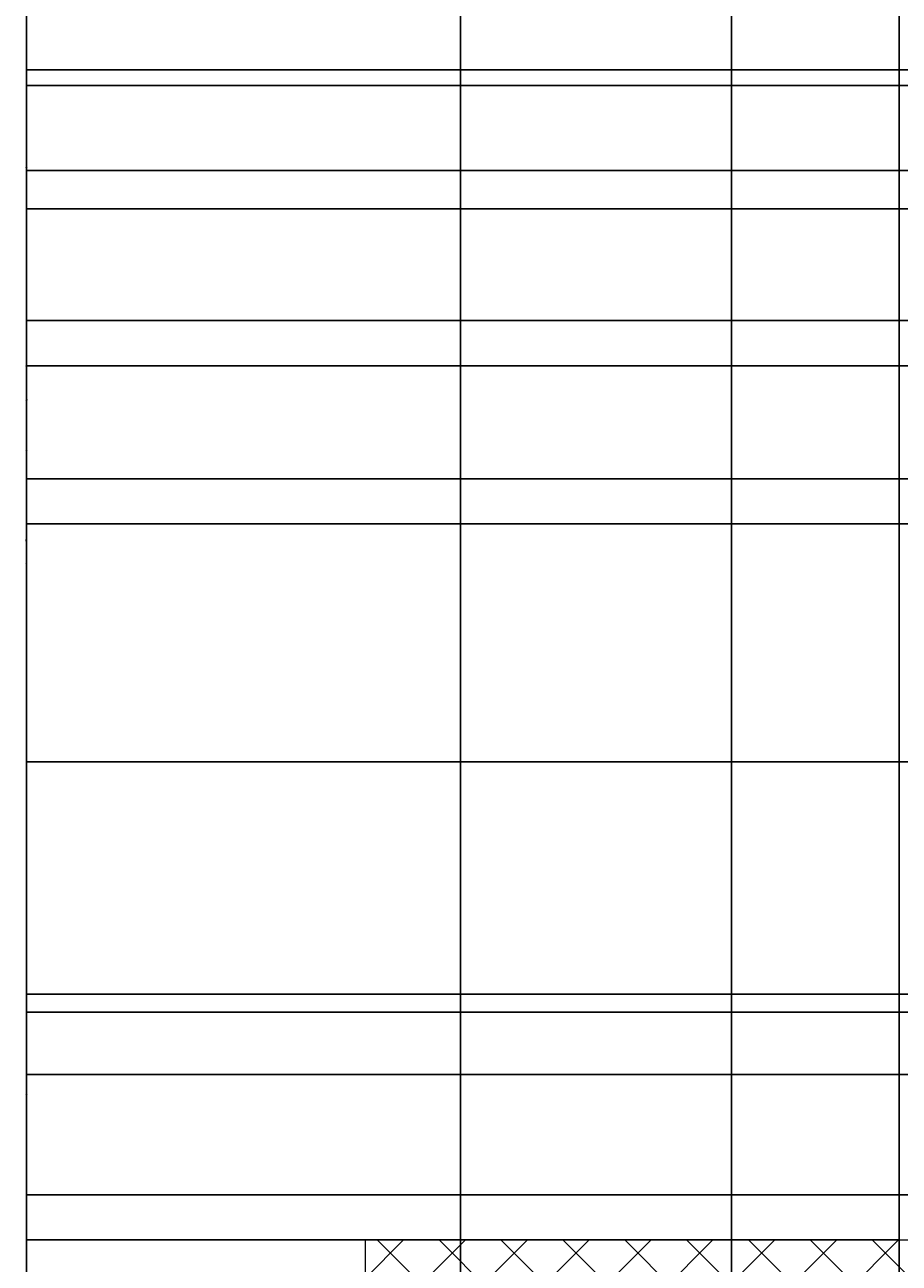
# Model space of a CAD drawing. Units: inches. Extents: x 818 to 1898, y 976 to 2364.
# Tile 2 of 96: x 818 to 993, y 1198 to 1446. Entities that reach past the tile are written whole.
import ezdxf

# ---------------------------------------------------------------- set-up
doc = ezdxf.new("R2010")
doc.units = ezdxf.units.IN
doc.header["$LTSCALE"] = 5
doc.header["$MEASUREMENT"] = 0
for name, color, linetype, lineweight in [('A-ANNO-DIMS', 2, 'Continuous', 18), ('C-PAVE-PATT', 8, 'Continuous', 9), ('L-PAVE', 8, 'Continuous', 18)]:
    doc.layers.add(name, color=color, linetype=linetype, lineweight=lineweight)
doc.styles.get("Standard").update_dxf_attribs({"font": 'arial.ttf'})
doc.dimstyles.get("Standard").update_dxf_attribs({"dimtxt": 0.18, "dimasz": 0.18, "dimexe": 0.18, "dimexo": 0.0625, "dimgap": 0.09, "dimtad": 0, "dimtih": 1, "dimtoh": 1, "dimdec": 4, "dimzin": 0, "dimdsep": 46, "dimtxsty": 'Standard', "dimcen": 0.09, "dimadec": 0, "dimazin": 0, "dimtfac": 1, "dimtdec": 4, "dimtofl": 0, "dimtmove": 0, "dimatfit": 3, "dimfxl": 1, "dimtolj": 1, "dimtzin": 0, "dimarcsym": 0})

# ---------------------------------------------------------------- blocks, each defined once
blk = doc.blocks.new('*D59')
at = {"layer": 'A-ANNO-DIMS', "color": 0, "lineweight": -2, "ltscale": 5, "transparency": 16777216}
for p, q in [((1251.64, 2300.39), (818.03, 2300.39)), ((818.21, 2300.21), (818.21, 1669.95)), ((818.21, 1039.32), (818.21, 1669.59)), ((896.05, 1039.14), (818.03, 1039.14))]:
    blk.add_line(p, q, dxfattribs=at)
at = {"layer": 'A-ANNO-DIMS', "color": 0, "ltscale": 5, "transparency": 16777216}
for points in [[(818.18, 2300.21), (818.24, 2300.21), (818.21, 2300.39)], [(818.18, 1039.32), (818.24, 1039.32), (818.21, 1039.14)]]:
    blk.add_solid(points, dxfattribs=at)
at = {"layer": 'Defpoints', "color": 0, "ltscale": 5, "transparency": 16777216}
for p in [(818.21, 2300.39), (1251.71, 2300.39), (896.11, 1039.14)]:
    blk.add_point(p, dxfattribs=at)
at = {"layer": 'A-ANNO-DIMS', "color": 0, "ltscale": 5, "transparency": 16777216, "insert": (818.21, 1669.77), "char_height": 0.18, "attachment_point": 5}
blk.add_mtext('\\A1;1261.2', dxfattribs=at)
blk = doc.blocks.new('*D60')
at = {"layer": 'A-ANNO-DIMS', "color": 0, "lineweight": -2, "ltscale": 5, "transparency": 16777216}
for p, q in [((992.66, 2294.22), (818.03, 2294.22)), ((818.21, 2294.04), (818.21, 1748.77)), ((818.21, 1203.14), (818.21, 1748.41)), ((992.66, 1202.96), (818.03, 1202.96))]:
    blk.add_line(p, q, dxfattribs=at)
at = {"layer": 'A-ANNO-DIMS', "color": 0, "ltscale": 5, "transparency": 16777216}
for points in [[(818.18, 2294.04), (818.24, 2294.04), (818.21, 2294.22)], [(818.18, 1203.14), (818.24, 1203.14), (818.21, 1202.96)]]:
    blk.add_solid(points, dxfattribs=at)
at = {"layer": 'Defpoints', "color": 0, "ltscale": 5, "transparency": 16777216}
for p in [(818.21, 2294.22), (992.73, 2294.22), (992.73, 1202.96)]:
    blk.add_point(p, dxfattribs=at)
at = {"layer": 'A-ANNO-DIMS', "color": 0, "ltscale": 5, "transparency": 16777216, "insert": (818.21, 1748.59), "char_height": 0.18, "attachment_point": 5}
blk.add_mtext('\\A1;1091.3', dxfattribs=at)
blk = doc.blocks.new('*D63')
at = {"layer": 'A-ANNO-DIMS', "color": 0, "lineweight": -2, "ltscale": 5, "transparency": 16777216}
for p, q in [((1116.13, 1485.2), (818.03, 1485.2)), ((818.21, 1485.02), (818.21, 1360.77)), ((818.21, 1236.14), (818.21, 1360.4)), ((1116.13, 1235.96), (818.03, 1235.96))]:
    blk.add_line(p, q, dxfattribs=at)
at = {"layer": 'A-ANNO-DIMS', "color": 0, "ltscale": 5, "transparency": 16777216}
for points in [[(818.18, 1485.02), (818.24, 1485.02), (818.21, 1485.2)], [(818.18, 1236.14), (818.24, 1236.14), (818.21, 1235.96)]]:
    blk.add_solid(points, dxfattribs=at)
at = {"layer": 'Defpoints', "color": 0, "ltscale": 5, "transparency": 16777216}
for p in [(818.21, 1485.2), (1116.19, 1485.2), (1116.19, 1235.96)]:
    blk.add_point(p, dxfattribs=at)
at = {"layer": 'A-ANNO-DIMS', "color": 0, "ltscale": 5, "transparency": 16777216, "insert": (818.21, 1360.58), "char_height": 0.18, "attachment_point": 5}
blk.add_mtext('\\A1;249.24', dxfattribs=at)
blk = doc.blocks.new('*D77')
at = {"layer": 'A-ANNO-DIMS', "color": 0, "lineweight": -2, "ltscale": 5, "transparency": 16777216}
for p, q in [((992.73, 1202.9), (992.73, 975.66)), ((896.11, 1104.9), (896.11, 975.66)), ((896.29, 975.84), (944.04, 975.84)), ((992.55, 975.84), (944.8, 975.84))]:
    blk.add_line(p, q, dxfattribs=at)
at = {"layer": 'A-ANNO-DIMS', "color": 0, "ltscale": 5, "transparency": 16777216}
for points in [[(896.29, 975.87), (896.29, 975.81), (896.11, 975.84)], [(992.55, 975.87), (992.55, 975.81), (992.73, 975.84)]]:
    blk.add_solid(points, dxfattribs=at)
at = {"layer": 'Defpoints', "color": 0, "ltscale": 5, "transparency": 16777216}
for p in [(992.73, 1202.96), (896.11, 1104.97), (992.73, 975.84)]:
    blk.add_point(p, dxfattribs=at)
at = {"layer": 'A-ANNO-DIMS', "color": 0, "ltscale": 5, "transparency": 16777216, "insert": (944.42, 975.84), "char_height": 0.18, "attachment_point": 5}
blk.add_mtext('\\A1;96.61', dxfattribs=at)
blk = doc.blocks.new('*D79')
at = {"layer": 'A-ANNO-DIMS', "color": 0, "lineweight": -2, "ltscale": 5, "transparency": 16777216}
for p, q in [((992.73, 1203.03), (992.73, 2363.87)), ((992.91, 2363.69), (1032.01, 2363.69)), ((1071.55, 2363.69), (1032.44, 2363.69)), ((1071.73, 1203.03), (1071.73, 2363.87))]:
    blk.add_line(p, q, dxfattribs=at)
at = {"layer": 'A-ANNO-DIMS', "color": 0, "ltscale": 5, "transparency": 16777216}
for points in [[(992.91, 2363.72), (992.91, 2363.66), (992.73, 2363.69)], [(1071.55, 2363.72), (1071.55, 2363.66), (1071.73, 2363.69)]]:
    blk.add_solid(points, dxfattribs=at)
at = {"layer": 'Defpoints', "color": 0, "ltscale": 5, "transparency": 16777216}
for p in [(1071.73, 2363.69), (992.73, 1202.96), (1071.73, 1202.96)]:
    blk.add_point(p, dxfattribs=at)
at = {"layer": 'A-ANNO-DIMS', "color": 0, "ltscale": 5, "transparency": 16777216, "insert": (1032.23, 2363.69), "char_height": 0.18, "attachment_point": 5}
blk.add_mtext('\\A1;79', dxfattribs=at)
blk = doc.blocks.new('*D81')
at = {"layer": 'A-ANNO-DIMS', "color": 0, "lineweight": -2, "ltscale": 5, "transparency": 16777216}
for p, q in [((1116.13, 1235.96), (818.03, 1235.96)), ((818.21, 1235.78), (818.21, 1224.14)), ((818.21, 1212.14), (818.21, 1223.78)), ((1083.66, 1211.96), (818.03, 1211.96))]:
    blk.add_line(p, q, dxfattribs=at)
at = {"layer": 'A-ANNO-DIMS', "color": 0, "ltscale": 5, "transparency": 16777216}
for points in [[(818.18, 1235.78), (818.24, 1235.78), (818.21, 1235.96)], [(818.18, 1212.14), (818.24, 1212.14), (818.21, 1211.96)]]:
    blk.add_solid(points, dxfattribs=at)
at = {"layer": 'Defpoints', "color": 0, "ltscale": 5, "transparency": 16777216}
for p in [(1116.19, 1235.96), (818.21, 1211.96), (1083.73, 1211.96)]:
    blk.add_point(p, dxfattribs=at)
at = {"layer": 'A-ANNO-DIMS', "color": 0, "ltscale": 5, "transparency": 16777216, "insert": (818.21, 1223.96), "char_height": 0.18, "attachment_point": 5}
blk.add_mtext('\\A1;24', dxfattribs=at)
blk = doc.blocks.new('*D90')
at = {"layer": 'A-ANNO-DIMS', "color": 0, "lineweight": -2, "ltscale": 5, "transparency": 16777216}
for p, q in [((904.95, 1071.12), (904.95, 2363.87)), ((905.13, 2363.69), (931.67, 2363.69)), ((958.99, 2363.69), (932.45, 2363.69)), ((959.17, 1071.12), (959.17, 2363.87))]:
    blk.add_line(p, q, dxfattribs=at)
at = {"layer": 'A-ANNO-DIMS', "color": 0, "ltscale": 5, "transparency": 16777216}
for points in [[(905.13, 2363.72), (905.13, 2363.66), (904.95, 2363.69)], [(958.99, 2363.72), (958.99, 2363.66), (959.17, 2363.69)]]:
    blk.add_solid(points, dxfattribs=at)
at = {"layer": 'Defpoints', "color": 0, "ltscale": 5, "transparency": 16777216}
for p in [(959.17, 2363.69), (904.95, 1071.06), (959.17, 1071.06)]:
    blk.add_point(p, dxfattribs=at)
at = {"layer": 'A-ANNO-DIMS', "color": 0, "ltscale": 5, "transparency": 16777216, "insert": (932.06, 2363.69), "char_height": 0.18, "attachment_point": 5}
blk.add_mtext('\\A1;54.22', dxfattribs=at)
blk = doc.blocks.new('*D91')
at = {"layer": 'A-ANNO-DIMS', "color": 0, "lineweight": -2, "ltscale": 5, "transparency": 16777216}
for p, q in [((959.17, 1071.12), (959.17, 2363.87)), ((959.35, 2363.69), (985.8, 2363.69)), ((1013.04, 2363.69), (986.59, 2363.69)), ((1013.22, 1071.12), (1013.22, 2363.87))]:
    blk.add_line(p, q, dxfattribs=at)
at = {"layer": 'A-ANNO-DIMS', "color": 0, "ltscale": 5, "transparency": 16777216}
for points in [[(959.35, 2363.72), (959.35, 2363.66), (959.17, 2363.69)], [(1013.04, 2363.72), (1013.04, 2363.66), (1013.22, 2363.69)]]:
    blk.add_solid(points, dxfattribs=at)
at = {"layer": 'Defpoints', "color": 0, "ltscale": 5, "transparency": 16777216}
for p in [(1013.22, 2363.69), (959.17, 1071.06), (1013.22, 1071.06)]:
    blk.add_point(p, dxfattribs=at)
at = {"layer": 'A-ANNO-DIMS', "color": 0, "ltscale": 5, "transparency": 16777216, "insert": (986.2, 2363.69), "char_height": 0.18, "attachment_point": 5}
blk.add_mtext('\\A1;54.04', dxfattribs=at)
blk = doc.blocks.new('*D108')
at = {"layer": 'A-ANNO-DIMS', "color": 0, "lineweight": -2, "ltscale": 5, "transparency": 16777216}
for p, q in [((1131.74, 1436.86), (818.03, 1436.86)), ((818.21, 1436.68), (818.21, 1342.84)), ((818.21, 1248.64), (818.21, 1342.48)), ((1164.49, 1248.46), (818.03, 1248.46))]:
    blk.add_line(p, q, dxfattribs=at)
at = {"layer": 'A-ANNO-DIMS', "color": 0, "ltscale": 5, "transparency": 16777216}
for points in [[(818.18, 1436.68), (818.24, 1436.68), (818.21, 1436.86)], [(818.18, 1248.64), (818.24, 1248.64), (818.21, 1248.46)]]:
    blk.add_solid(points, dxfattribs=at)
at = {"layer": 'Defpoints', "color": 0, "ltscale": 5, "transparency": 16777216}
for p in [(818.21, 1436.86), (1131.8, 1436.86), (1164.56, 1248.46)]:
    blk.add_point(p, dxfattribs=at)
at = {"layer": 'A-ANNO-DIMS', "color": 0, "ltscale": 5, "transparency": 16777216, "insert": (818.21, 1342.66), "char_height": 0.18, "attachment_point": 5}
blk.add_mtext('\\A1;188.4', dxfattribs=at)
blk = doc.blocks.new('*D115')
at = {"layer": 'A-ANNO-DIMS', "color": 0, "lineweight": -2, "ltscale": 5, "transparency": 16777216}
for p, q in [((1766.29, 1377.66), (818.03, 1377.66)), ((818.21, 1377.48), (818.21, 1338.26)), ((818.21, 1298.68), (818.21, 1337.9)), ((1766.29, 1298.5), (818.03, 1298.5))]:
    blk.add_line(p, q, dxfattribs=at)
at = {"layer": 'A-ANNO-DIMS', "color": 0, "ltscale": 5, "transparency": 16777216}
for points in [[(818.18, 1377.48), (818.24, 1377.48), (818.21, 1377.66)], [(818.18, 1298.68), (818.24, 1298.68), (818.21, 1298.5)]]:
    blk.add_solid(points, dxfattribs=at)
at = {"layer": 'Defpoints', "color": 0, "ltscale": 5, "transparency": 16777216}
for p in [(818.21, 1377.66), (1766.35, 1377.66), (1766.35, 1298.5)]:
    blk.add_point(p, dxfattribs=at)
at = {"layer": 'A-ANNO-DIMS', "color": 0, "ltscale": 5, "transparency": 16777216, "insert": (818.21, 1338.08), "char_height": 0.18, "attachment_point": 5}
blk.add_mtext('\\A1;79.15', dxfattribs=at)
blk = doc.blocks.new('*D116')
at = {"layer": 'A-ANNO-DIMS', "color": 0, "lineweight": -2, "ltscale": 5, "transparency": 16777216}
for p, q in [((1766.29, 1456.81), (818.03, 1456.81)), ((818.21, 1456.63), (818.21, 1417.41)), ((818.21, 1377.84), (818.21, 1417.05)), ((1766.29, 1377.66), (818.03, 1377.66))]:
    blk.add_line(p, q, dxfattribs=at)
at = {"layer": 'A-ANNO-DIMS', "color": 0, "ltscale": 5, "transparency": 16777216}
for points in [[(818.18, 1456.63), (818.24, 1456.63), (818.21, 1456.81)], [(818.18, 1377.84), (818.24, 1377.84), (818.21, 1377.66)]]:
    blk.add_solid(points, dxfattribs=at)
at = {"layer": 'Defpoints', "color": 0, "ltscale": 5, "transparency": 16777216}
for p in [(818.21, 1456.81), (1766.35, 1456.81), (1766.35, 1377.66)]:
    blk.add_point(p, dxfattribs=at)
at = {"layer": 'A-ANNO-DIMS', "color": 0, "ltscale": 5, "transparency": 16777216, "insert": (818.21, 1417.23), "char_height": 0.18, "attachment_point": 5}
blk.add_mtext('\\A1;79.15', dxfattribs=at)
blk = doc.blocks.new('*D127')
at = {"layer": 'A-ANNO-DIMS', "color": 0, "lineweight": -2, "ltscale": 5, "transparency": 16777216}
for p, q in [((1035.31, 1252.02), (818.03, 1252.02)), ((818.21, 1251.84), (818.21, 1232.18)), ((818.21, 1212.14), (818.21, 1231.81)), ((1001.66, 1211.96), (818.03, 1211.96))]:
    blk.add_line(p, q, dxfattribs=at)
at = {"layer": 'A-ANNO-DIMS', "color": 0, "ltscale": 5, "transparency": 16777216}
for points in [[(818.18, 1251.84), (818.24, 1251.84), (818.21, 1252.02)], [(818.18, 1212.14), (818.24, 1212.14), (818.21, 1211.96)]]:
    blk.add_solid(points, dxfattribs=at)
at = {"layer": 'Defpoints', "color": 0, "ltscale": 5, "transparency": 16777216}
for p in [(818.21, 1252.02), (1035.38, 1252.02), (1001.73, 1211.96)]:
    blk.add_point(p, dxfattribs=at)
at = {"layer": 'A-ANNO-DIMS', "color": 0, "ltscale": 5, "transparency": 16777216, "insert": (818.21, 1231.99), "char_height": 0.18, "attachment_point": 5}
blk.add_mtext('\\A1;40.06', dxfattribs=at)
blk = doc.blocks.new('*D128')
at = {"layer": 'A-ANNO-DIMS', "color": 0, "lineweight": -2, "ltscale": 5, "transparency": 16777216}
for p, q in [((1044.78, 1433.67), (818.03, 1433.67)), ((818.21, 1433.49), (818.21, 1343.03)), ((818.21, 1252.2), (818.21, 1342.66)), ((1035.31, 1252.02), (818.03, 1252.02))]:
    blk.add_line(p, q, dxfattribs=at)
at = {"layer": 'A-ANNO-DIMS', "color": 0, "ltscale": 5, "transparency": 16777216}
for points in [[(818.18, 1433.49), (818.24, 1433.49), (818.21, 1433.67)], [(818.18, 1252.2), (818.24, 1252.2), (818.21, 1252.02)]]:
    blk.add_solid(points, dxfattribs=at)
at = {"layer": 'Defpoints', "color": 0, "ltscale": 5, "transparency": 16777216}
for p in [(818.21, 1433.67), (1044.85, 1433.67), (1035.38, 1252.02)]:
    blk.add_point(p, dxfattribs=at)
at = {"layer": 'A-ANNO-DIMS', "color": 0, "ltscale": 5, "transparency": 16777216, "insert": (818.21, 1342.85), "char_height": 0.18, "attachment_point": 5}
blk.add_mtext('\\A1;181.64', dxfattribs=at)
blk = doc.blocks.new('*D129')
at = {"layer": 'A-ANNO-DIMS', "color": 0, "lineweight": -2, "ltscale": 5, "transparency": 16777216}
for p, q in [((1044.78, 1608.51), (818.03, 1608.51)), ((818.21, 1608.33), (818.21, 1521.27)), ((818.21, 1433.85), (818.21, 1520.91)), ((1044.78, 1433.67), (818.03, 1433.67))]:
    blk.add_line(p, q, dxfattribs=at)
at = {"layer": 'A-ANNO-DIMS', "color": 0, "ltscale": 5, "transparency": 16777216}
for points in [[(818.18, 1608.33), (818.24, 1608.33), (818.21, 1608.51)], [(818.18, 1433.85), (818.24, 1433.85), (818.21, 1433.67)]]:
    blk.add_solid(points, dxfattribs=at)
at = {"layer": 'Defpoints', "color": 0, "ltscale": 5, "transparency": 16777216}
for p in [(818.21, 1608.51), (1044.85, 1608.51), (1044.85, 1433.67)]:
    blk.add_point(p, dxfattribs=at)
at = {"layer": 'A-ANNO-DIMS', "color": 0, "ltscale": 5, "transparency": 16777216, "insert": (818.21, 1521.09), "char_height": 0.18, "attachment_point": 5}
blk.add_mtext('\\A1;174.84', dxfattribs=at)
blk = doc.blocks.new('*D171')
at = {"layer": 'A-ANNO-DIMS', "color": 0, "lineweight": -2, "ltscale": 5, "transparency": 16777216}
for p, q in [((1616.66, 1386.69), (818.03, 1386.69)), ((818.21, 1386.51), (818.21, 1371.06)), ((818.21, 1355.26), (818.21, 1370.7)), ((1616.66, 1355.08), (818.03, 1355.08))]:
    blk.add_line(p, q, dxfattribs=at)
at = {"layer": 'A-ANNO-DIMS', "color": 0, "ltscale": 5, "transparency": 16777216}
for points in [[(818.18, 1386.51), (818.24, 1386.51), (818.21, 1386.69)], [(818.18, 1355.26), (818.24, 1355.26), (818.21, 1355.08)]]:
    blk.add_solid(points, dxfattribs=at)
at = {"layer": 'Defpoints', "color": 0, "ltscale": 5, "transparency": 16777216}
for p in [(818.21, 1386.69), (1616.73, 1386.69), (1616.73, 1355.08)]:
    blk.add_point(p, dxfattribs=at)
at = {"layer": 'A-ANNO-DIMS', "color": 0, "ltscale": 5, "transparency": 16777216, "insert": (818.21, 1370.88), "char_height": 0.18, "attachment_point": 5}
blk.add_mtext('\\A1;31.61', dxfattribs=at)
blk = doc.blocks.new('*D172')
at = {"layer": 'A-ANNO-DIMS', "color": 0, "lineweight": -2, "ltscale": 5, "transparency": 16777216}
for p, q in [((1616.66, 1416.69), (818.03, 1416.69)), ((818.21, 1416.51), (818.21, 1401.87)), ((818.21, 1386.87), (818.21, 1401.5)), ((1616.66, 1386.69), (818.03, 1386.69))]:
    blk.add_line(p, q, dxfattribs=at)
at = {"layer": 'A-ANNO-DIMS', "color": 0, "ltscale": 5, "transparency": 16777216}
for points in [[(818.18, 1416.51), (818.24, 1416.51), (818.21, 1416.69)], [(818.18, 1386.87), (818.24, 1386.87), (818.21, 1386.69)]]:
    blk.add_solid(points, dxfattribs=at)
at = {"layer": 'Defpoints', "color": 0, "ltscale": 5, "transparency": 16777216}
for p in [(818.21, 1416.69), (1616.73, 1416.69), (1616.73, 1386.69)]:
    blk.add_point(p, dxfattribs=at)
at = {"layer": 'A-ANNO-DIMS', "color": 0, "ltscale": 5, "transparency": 16777216, "insert": (818.21, 1401.69), "char_height": 0.18, "attachment_point": 5}
blk.add_mtext('\\A1;30', dxfattribs=at)
blk = doc.blocks.new('*D190')
at = {"layer": 'A-ANNO-DIMS', "color": 0, "lineweight": -2, "ltscale": 5, "transparency": 16777216}
for p, q in [((1430.66, 1409.05), (818.03, 1409.05)), ((818.21, 1408.87), (818.21, 1377.75)), ((818.21, 1346.26), (818.21, 1377.38)), ((1430.66, 1346.08), (818.03, 1346.08))]:
    blk.add_line(p, q, dxfattribs=at)
at = {"layer": 'A-ANNO-DIMS', "color": 0, "ltscale": 5, "transparency": 16777216}
for points in [[(818.18, 1408.87), (818.24, 1408.87), (818.21, 1409.05)], [(818.18, 1346.26), (818.24, 1346.26), (818.21, 1346.08)]]:
    blk.add_solid(points, dxfattribs=at)
at = {"layer": 'Defpoints', "color": 0, "ltscale": 5, "transparency": 16777216}
for p in [(818.21, 1409.05), (1430.73, 1409.05), (1430.73, 1346.08)]:
    blk.add_point(p, dxfattribs=at)
at = {"layer": 'A-ANNO-DIMS', "color": 0, "ltscale": 5, "transparency": 16777216, "insert": (818.21, 1377.57), "char_height": 0.18, "attachment_point": 5}
blk.add_mtext('\\A1;62.97', dxfattribs=at)

msp = doc.modelspace()

# ---------------------------------------------------------------- hatches: boundary and pattern name
at = {"layer": 'C-PAVE-PATT', "ltscale": 5}
h = msp.add_hatch(dxfattribs=at)
h.set_pattern_fill('ANSI37', color=256, scale=70)
h.paths.add_polyline_path([(1071.7251, 1202.9642), (885.9457, 1202.9642), (885.9457, 1167.3717), (1059.7252, 1167.3717, 0.41421356), (1071.7251, 1179.3717)])
h.paths.add_polyline_path([(1828.9123, 1202.9642), (1430.7251, 1202.9642), (1430.7251, 1179.3717, 0.41421356), (1442.7252, 1167.3717), (1828.9123, 1167.3717)])

# ---------------------------------------------------------------- linework, layer by layer
at = {"layer": 'L-PAVE', "ltscale": 5}
msp.add_lwpolyline([(885.9457, 1202.9642), (1071.7251, 1202.9642), (1071.7251, 1179.3717, -0.41421356), (1059.7252, 1167.3717), (885.9457, 1167.3717)], format="xyb", close=True, dxfattribs=at)

# ---------------------------------------------------------------- dimensions: what is measured, and where the dimension line sits
at = {"layer": 'A-ANNO-DIMS', "ltscale": 5}
for base, p1, p2, override, picture, middle in [((959.1737, 2363.6929), (904.9504, 1071.0552), (959.1737, 1071.0552), {"dimdec": 2, "dimlfac": 1, "dimrnd": 0, "dimzin": 0, "dimdsep": 46, "dimlunit": 2}, '*D90', (932.062, 2363.6929)), ((1013.2176, 2363.6929), (959.1737, 1071.0552), (1013.2176, 1071.0552), {"dimdec": 2, "dimlfac": 1, "dimrnd": 0, "dimzin": 0, "dimdsep": 46, "dimlunit": 2}, '*D91', (986.1956, 2363.6929)), ((1071.7251, 2363.6929), (992.7251, 1202.9642), (1071.7251, 1202.9642), {"dimdec": 0, "dimlfac": 1, "dimrnd": 0, "dimzin": 0, "dimdsep": 46, "dimlunit": 2}, '*D79', (1032.2251, 2363.6929)), ((992.7251, 975.8433), (896.1138, 1104.9672), (992.7251, 1202.9642), {"dimdec": 2, "dimlfac": 1, "dimrnd": 0, "dimzin": 0, "dimdsep": 46, "dimlunit": 2}, '*D77', (944.4195, 975.8433))]:
    dim = msp.add_linear_dim(base=base, p1=p1, p2=p2, dimstyle='Standard', override=override, dxfattribs=at)
    dim.commit()
    dim.dimension.update_dxf_attribs({"geometry": picture, "text_midpoint": middle})
for base, p1, p2, override, picture, middle in [((818.2059, 2300.3929), (896.1138, 1039.1433), (1251.7057, 2300.3929), {"dimdec": 1, "dimlfac": 1, "dimrnd": 0, "dimzin": 0, "dimdsep": 46, "dimlunit": 2}, '*D59', (818.2059, 1669.7681)), ((818.2059, 2294.2171), (992.7251, 1202.9642), (992.7251, 2294.2171), {"dimdec": 1, "dimlfac": 1, "dimrnd": 0, "dimzin": 0, "dimdsep": 46, "dimlunit": 2}, '*D60', (818.2059, 1748.5907)), ((818.2059, 1608.5116), (1044.8463, 1433.6672), (1044.8463, 1608.5116), {"dimdec": 2, "dimlfac": 1, "dimrnd": 0, "dimzin": 0, "dimdsep": 46, "dimlunit": 2}, '*D129', (818.2059, 1521.0894)), ((818.2059, 1485.2035), (1116.1882, 1235.9642), (1116.1882, 1485.2035), {"dimdec": 2, "dimlfac": 1, "dimrnd": 0, "dimzin": 0, "dimdsep": 46, "dimlunit": 2}, '*D63', (818.2059, 1360.5839)), ((818.2059, 1456.8088), (1766.3524, 1377.6564), (1766.3524, 1456.8088), {"dimdec": 2, "dimlfac": 1, "dimrnd": 0, "dimzin": 0, "dimdsep": 46, "dimlunit": 2}, '*D116', (818.2059, 1417.2326)), ((818.2059, 1436.8613), (1164.5571, 1248.4622), (1131.7984, 1436.8613), {"dimdec": 1, "dimlfac": 1, "dimrnd": 0, "dimzin": 0, "dimdsep": 46, "dimlunit": 2}, '*D108', (818.2059, 1342.6618)), ((818.2059, 1433.6672), (1035.3768, 1252.0242), (1044.8463, 1433.6672), {"dimdec": 2, "dimlfac": 1, "dimrnd": 0, "dimzin": 0, "dimdsep": 46, "dimlunit": 2}, '*D128', (818.2059, 1342.8457)), ((818.2059, 1416.6857), (1616.7251, 1386.6857), (1616.7251, 1416.6857), {"dimdec": 0, "dimlfac": 1, "dimrnd": 0, "dimzin": 0, "dimdsep": 46, "dimlunit": 2}, '*D172', (818.2059, 1401.6857)), ((818.2059, 1409.0522), (1430.7251, 1346.0782), (1430.7251, 1409.0522), {"dimdec": 2, "dimlfac": 1, "dimrnd": 0, "dimzin": 0, "dimdsep": 46, "dimlunit": 2}, '*D190', (818.2059, 1377.5652)), ((818.2059, 1386.6857), (1616.7251, 1355.0782), (1616.7251, 1386.6857), {"dimdec": 2, "dimlfac": 1, "dimrnd": 0, "dimzin": 0, "dimdsep": 46, "dimlunit": 2}, '*D171', (818.2059, 1370.882)), ((818.2059, 1377.6564), (1766.3524, 1298.5041), (1766.3524, 1377.6564), {"dimdec": 2, "dimlfac": 1, "dimrnd": 0, "dimzin": 0, "dimdsep": 46, "dimlunit": 2}, '*D115', (818.2059, 1338.0803)), ((818.2059, 1252.0242), (1001.7251, 1211.9642), (1035.3768, 1252.0242), {"dimdec": 2, "dimlfac": 1, "dimrnd": 0, "dimzin": 0, "dimdsep": 46, "dimlunit": 2}, '*D127', (818.2059, 1231.9942)), ((818.2059, 1211.9642), (1116.1882, 1235.9642), (1083.7251, 1211.9642), {"dimdec": 0, "dimlfac": 1, "dimrnd": 0, "dimzin": 0, "dimdsep": 46, "dimlunit": 2}, '*D81', (818.2059, 1223.9642))]:
    dim = msp.add_linear_dim(base=base, p1=p1, p2=p2, angle=90, dimstyle='Standard', override=override, dxfattribs=at)
    dim.commit()
    dim.dimension.update_dxf_attribs({"geometry": picture, "text_midpoint": middle})

doc.saveas('drawing.dxf')
